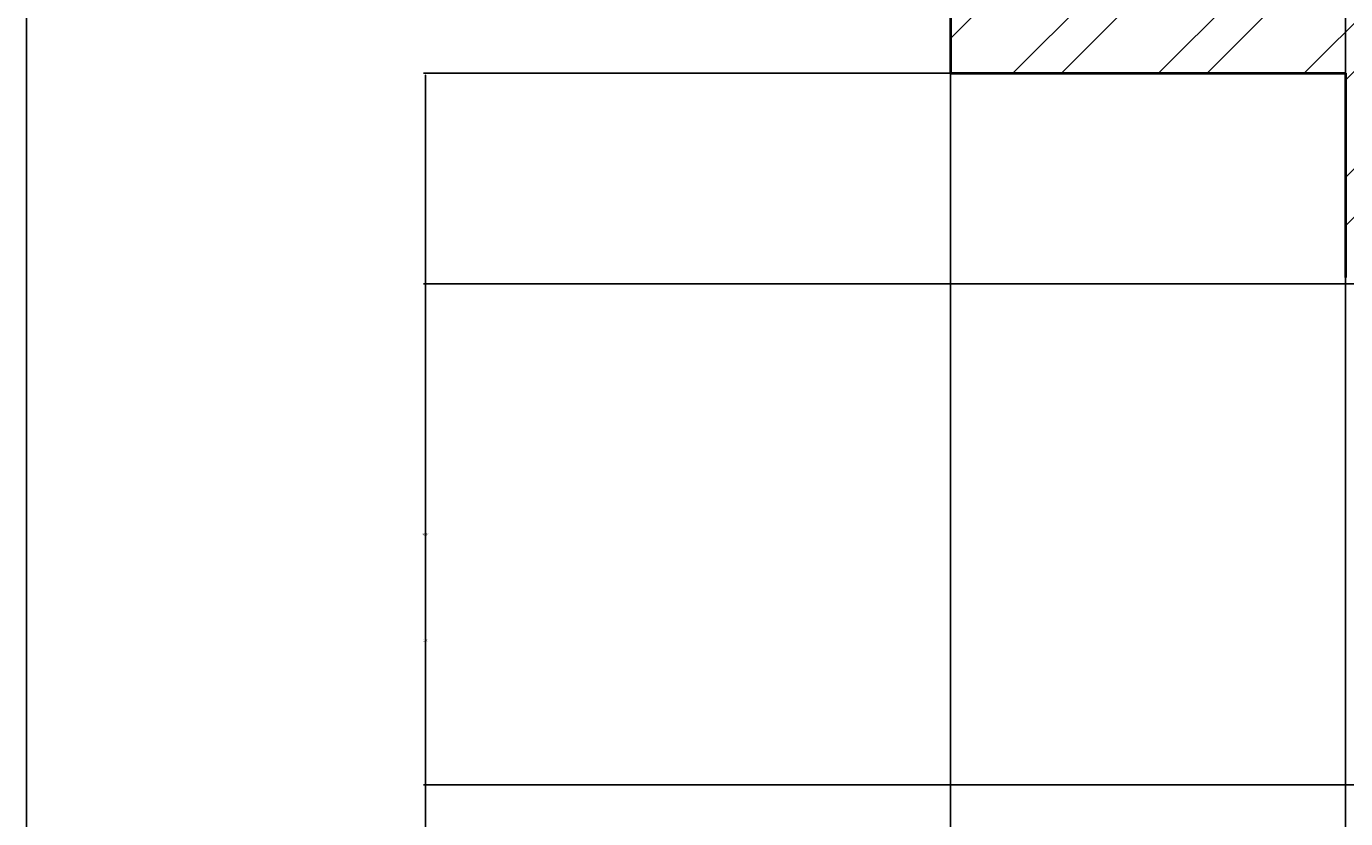
# Model space of a CAD drawing. Units: inches. Extents: x 1601 to 2297, y 1496 to 2631.
# Tile 11 of 57: x 1601 to 1723, y 2067 to 2141. Entities that reach past the tile are written whole.
import ezdxf

# ---------------------------------------------------------------- set-up
doc = ezdxf.new("R2010")
doc.units = ezdxf.units.IN
for name, color, linetype, lineweight in [('A-ANNO-DIMS', 2, 'Continuous', 18), ('A-ANNO-TTLB', 7, 'Continuous', 25), ('A-WALL', 7, 'Continuous', 40), ('A-WALL-PATT', 215, 'Continuous', 13)]:
    doc.layers.add(name, color=color, linetype=linetype, lineweight=lineweight)
doc.styles.get("Standard").update_dxf_attribs({"font": 'arial.ttf'})
doc.dimstyles.get("Standard").update_dxf_attribs({"dimtxt": 0.18, "dimasz": 0.18, "dimexe": 0.18, "dimexo": 0.0625, "dimgap": 0.09, "dimtad": 0, "dimtih": 1, "dimtoh": 1, "dimdec": 4, "dimzin": 0, "dimdsep": 46, "dimtxsty": 'Standard', "dimcen": 0.09, "dimadec": 0, "dimazin": 0, "dimtfac": 1, "dimtdec": 4, "dimtofl": 0, "dimtmove": 0, "dimatfit": 3, "dimfxl": 1, "dimtolj": 1, "dimtzin": 0, "dimarcsym": 0})

# ---------------------------------------------------------------- blocks, each defined once
blk = doc.blocks.new('*D31')
at = {"layer": 'A-ANNO-DIMS', "color": 0, "lineweight": -2, "transparency": 16777216}
for p, q in [((1685.97, 2136.33), (1637.31, 2136.33)), ((1637.49, 2136.15), (1637.49, 2084.01)), ((1637.49, 2031.51), (1637.49, 2083.64)), ((1685.97, 2031.33), (1637.31, 2031.33))]:
    blk.add_line(p, q, dxfattribs=at)
at = {"layer": 'A-ANNO-DIMS', "color": 0, "transparency": 16777216}
for points in [[(1637.46, 2136.15), (1637.52, 2136.15), (1637.49, 2136.33)], [(1637.46, 2031.51), (1637.52, 2031.51), (1637.49, 2031.33)]]:
    blk.add_solid(points, dxfattribs=at)
at = {"layer": 'Defpoints', "color": 0, "transparency": 16777216}
for p in [(1637.49, 2136.33), (1686.04, 2136.33), (1686.04, 2031.33)]:
    blk.add_point(p, dxfattribs=at)
at = {"layer": 'A-ANNO-DIMS', "color": 0, "transparency": 16777216, "insert": (1637.49, 2083.83), "char_height": 0.18, "attachment_point": 5}
blk.add_mtext('\\A1;105', dxfattribs=at)
blk = doc.blocks.new('*D32')
at = {"layer": 'A-ANNO-DIMS', "color": 0, "lineweight": -2, "transparency": 16777216}
for p, q in [((1686.04, 2031.39), (1686.04, 2581.06)), ((1722.57, 2031.39), (1722.57, 2581.06)), ((1686.22, 2580.88), (1703.91, 2580.88)), ((1722.39, 2580.88), (1704.7, 2580.88))]:
    blk.add_line(p, q, dxfattribs=at)
at = {"layer": 'A-ANNO-DIMS', "color": 0, "transparency": 16777216}
for points in [[(1686.22, 2580.91), (1686.22, 2580.85), (1686.04, 2580.88)], [(1722.39, 2580.91), (1722.39, 2580.85), (1722.57, 2580.88)]]:
    blk.add_solid(points, dxfattribs=at)
at = {"layer": 'Defpoints', "color": 0, "transparency": 16777216}
for p in [(1722.57, 2580.88), (1686.04, 2031.33), (1722.57, 2031.33)]:
    blk.add_point(p, dxfattribs=at)
at = {"layer": 'A-ANNO-DIMS', "color": 0, "transparency": 16777216, "insert": (1704.3, 2580.88), "char_height": 0.18, "attachment_point": 5}
blk.add_mtext('\\A1;36.53', dxfattribs=at)
blk = doc.blocks.new('*D36')
at = {"layer": 'A-ANNO-DIMS', "color": 0, "lineweight": -2, "transparency": 16777216}
for p, q in [((1686.04, 1635.39), (1686.04, 2581.06)), ((1739.33, 1635.39), (1739.33, 2581.06)), ((1686.22, 2580.88), (1712.36, 2580.88)), ((1739.15, 2580.88), (1713.01, 2580.88))]:
    blk.add_line(p, q, dxfattribs=at)
at = {"layer": 'A-ANNO-DIMS', "color": 0, "transparency": 16777216}
for points in [[(1686.22, 2580.91), (1686.22, 2580.85), (1686.04, 2580.88)], [(1739.15, 2580.91), (1739.15, 2580.85), (1739.33, 2580.88)]]:
    blk.add_solid(points, dxfattribs=at)
at = {"layer": 'Defpoints', "color": 0, "transparency": 16777216}
for p in [(1739.33, 2580.88), (1686.04, 1635.33), (1739.33, 1635.33)]:
    blk.add_point(p, dxfattribs=at)
at = {"layer": 'A-ANNO-DIMS', "color": 0, "transparency": 16777216, "insert": (1712.69, 2580.88), "char_height": 0.18, "attachment_point": 5}
blk.add_mtext('\\A1;53.3', dxfattribs=at)
blk = doc.blocks.new('*D44')
at = {"layer": 'A-ANNO-DIMS', "color": 0, "lineweight": -2, "transparency": 16777216}
for p, q in [((1958.97, 2116.84), (1637.31, 2116.84)), ((1637.49, 2116.66), (1637.49, 2093.85)), ((1637.49, 2070.67), (1637.49, 2093.48)), ((1958.97, 2070.49), (1637.31, 2070.49))]:
    blk.add_line(p, q, dxfattribs=at)
at = {"layer": 'A-ANNO-DIMS', "color": 0, "transparency": 16777216}
for points in [[(1637.46, 2116.66), (1637.52, 2116.66), (1637.49, 2116.84)], [(1637.46, 2070.67), (1637.52, 2070.67), (1637.49, 2070.49)]]:
    blk.add_solid(points, dxfattribs=at)
at = {"layer": 'Defpoints', "color": 0, "transparency": 16777216}
for p in [(1637.49, 2116.84), (1959.04, 2116.84), (1959.04, 2070.49)]:
    blk.add_point(p, dxfattribs=at)
at = {"layer": 'A-ANNO-DIMS', "color": 0, "transparency": 16777216, "insert": (1637.49, 2093.67), "char_height": 0.18, "attachment_point": 5}
blk.add_mtext('\\A1;46.34', dxfattribs=at)

msp = doc.modelspace()

# ---------------------------------------------------------------- hatches: boundary and pattern name
at = {"layer": 'A-WALL-PATT'}
h = msp.add_hatch(dxfattribs=at)
h.set_pattern_fill('ANSI32', color=256)
h.paths.add_polyline_path([(1973.9371, 2211.3254), (1893.0373, 2211.3254), (1893.0373, 2287.8254), (1884.6167, 2287.8254), (1884.6167, 2285.5754), (1884.6167, 2283.3254), (1888.5373, 2283.3254), (1888.5373, 2145.3254), (1695.0373, 2145.3254), (1695.0373, 2173.8724), (1690.5373, 2173.8724), (1686.0373, 2173.8724), (1686.0373, 2136.3254), (1722.5687, 2136.3254), (1722.5687, 2117.4352), (1731.5687, 2117.4352), (1731.5687, 2136.3254), (1893.0373, 2136.3254), (1893.0373, 2202.3254), (1959.0373, 2202.3254), (1959.0373, 2182.1303), (1968.0373, 2182.1303), (1968.0373, 2202.3254), (1973.9371, 2202.3254)])
h.paths.add_polyline_path([(2094.0373, 2274.6364), (2096.4294, 2274.6364), (2096.4294, 2276.8864), (2096.4294, 2279.1364), (2094.0373, 2279.1364), (2094.0373, 2290.8254), (2094.0373, 2295.3254), (2089.5373, 2295.3254), (2089.5373, 2230.8254), (2035.5373, 2230.8254), (2035.5373, 2299.8254), (2031.0373, 2299.8254), (2031.0373, 2211.3254), (2023.0065, 2211.3254), (2023.0065, 2202.3254), (2031.0373, 2202.3254), (2031.0373, 2140.8254), (1968.0373, 2140.8254), (1968.0373, 2145.9106), (1963.5373, 2145.9106), (1959.0373, 2145.9106), (1959.0373, 2116.839), (1963.5373, 2116.839), (1968.0373, 2116.839), (1968.0373, 2131.8254), (2031.0373, 2131.8254), (2031.0373, 2094.3254), (2031.0373, 2085.3254), (2031.0373, 2056.8254), (1968.0373, 2056.8254), (1968.0373, 2070.4947), (1963.5373, 2070.4947), (1959.0373, 2070.4947), (1959.0373, 2040.3029), (1968.0373, 2040.3029), (1968.0373, 2047.8254), (2031.0373, 2047.8254), (2031.0373, 1983.3254), (2031.0373, 1978.8254), (2021.1979, 1978.8254), (2021.1979, 1974.3254), (2031.0373, 1974.3254), (2031.0373, 1954.3528), (2035.5373, 1954.3528), (2035.5373, 1974.3254), (2035.5373, 1981.8254), (2055.5513, 1981.8254), (2055.5513, 1986.3254), (2035.5373, 1986.3254), (2035.5373, 2047.8254), (2040.0373, 2047.8254), (2040.0373, 2085.3254), (2040.0373, 2094.3254), (2040.0373, 2140.8254), (2035.5373, 2140.8254), (2035.5373, 2226.3254), (2089.5373, 2226.3254), (2094.0373, 2226.3254)])
h.paths.add_polyline_path([(2226.0373, 2230.8254), (2134.5373, 2230.8254), (2134.5373, 2233.5437), (2130.0373, 2233.5437), (2130.0373, 2226.3254), (2134.5373, 2226.3254), (2226.0373, 2226.3254)])
h.paths.add_polyline_path([(1807.1169, 1573.5395), (2055.0405, 1573.5395), (2055.0405, 1610.6322), (1807.1169, 1610.6322)], flags=9)
h.paths.add_polyline_path([(1841.1631, 1712.7967), (1870.3957, 1712.7967), (1870.3957, 1731.454), (1841.1631, 1731.454)], flags=9)
h.paths.add_polyline_path([(2144.3862, 1772.185), (2191.0233, 1772.185), (2191.0233, 1790.8423), (2144.3862, 1790.8423)], flags=9)
h.paths.add_polyline_path([(2143.0128, 1827.3312), (2177.9958, 1827.3312), (2177.9958, 1845.9886), (2143.0128, 1845.9886)], flags=9)
h.paths.add_polyline_path([(2041.2439, 1833.5691), (2070.8516, 1833.5691), (2070.8516, 1852.2264), (2041.2439, 1852.2264)], flags=9)
h.paths.add_polyline_path([(2097.2791, 1947.0598), (2134.2061, 1947.0598), (2134.2061, 1965.7171), (2097.2791, 1965.7171)], flags=9)
h.paths.add_polyline_path([(2214.995, 1904.3124), (2214.995, 1942.2899), (2196.3376, 1942.2899), (2196.3376, 1904.3124)], flags=9)
h.paths.add_polyline_path([(2186.6284, 2043.8031), (2219.7935, 2043.8031), (2219.7935, 2062.4605), (2186.6284, 2062.4605)], flags=9)
h.paths.add_polyline_path([(2064.0877, 2031.616), (2097.4949, 2031.616), (2097.4949, 2050.2734), (2064.0877, 2050.2734)], flags=9)
h.paths.add_polyline_path([(1973.1349, 1986.0688), (2008.4009, 1986.0688), (2008.4009, 2004.7261), (1973.1349, 2004.7261)], flags=25)
h.paths.add_polyline_path([(1976.3676, 2106.9635), (2005.7469, 2106.9635), (2005.7469, 2125.6209), (1976.3676, 2125.6209)], flags=25)
h.paths.add_polyline_path([(1991.7852, 2180.4863), (2027.0513, 2180.4863), (2027.0513, 2199.1437), (1991.7852, 2199.1437)], flags=25)
h.paths.add_polyline_path([(2106.1801, 2187.9359), (2152.2101, 2187.9359), (2152.2101, 2206.5932), (2106.1801, 2206.5932)], flags=9)
h.paths.add_polyline_path([(2148.6686, 2262.2542), (2182.318, 2262.2542), (2182.318, 2280.9115), (2148.6686, 2280.9115)], flags=9)
h.paths.add_polyline_path([(2041.6327, 2252.8147), (2071.2405, 2252.8147), (2071.2405, 2271.4721), (2041.6327, 2271.4721)], flags=25)
h.paths.add_polyline_path([(2063.9734, 2375.4265), (2100.9004, 2375.4265), (2100.9004, 2394.0839), (2063.9734, 2394.0839)], flags=9)
h.paths.add_polyline_path([(2216.4955, 2330.9748), (2216.4955, 2370.2654), (2197.8381, 2370.2654), (2197.8381, 2330.9748)], flags=9)
h.paths.add_polyline_path([(2179.1416, 2485.8687), (2212.3067, 2485.8687), (2212.3067, 2504.5261), (2179.1416, 2504.5261)], flags=9)
h.paths.add_polyline_path([(2078.7442, 2471.1516), (2112.1514, 2471.1516), (2112.1514, 2489.809), (2078.7442, 2489.809)], flags=9)
h.paths.add_polyline_path([(1915.9631, 2329.4668), (1952.8902, 2329.4668), (1952.8902, 2348.1241), (1915.9631, 2348.1241)], flags=9)
h.paths.add_polyline_path([(1904.3189, 2499.6709), (1940.4512, 2499.6709), (1940.4512, 2518.3282), (1904.3189, 2518.3282)], flags=9)
h.paths.add_polyline_path([(1892.3665, 2100.4595), (1925.6374, 2100.4595), (1925.6374, 2119.1169), (1892.3665, 2119.1169)], flags=9)
h.paths.add_polyline_path([(1909.2984, 1805.9631), (1946.2254, 1805.9631), (1946.2254, 1824.6205), (1909.2984, 1824.6205)], flags=9)
h.paths.add_polyline_path([(1934.6056, 1658.616), (1970.738, 1658.616), (1970.738, 1677.2733), (1934.6056, 1677.2733)], flags=9)
h.paths.add_polyline_path([(1711.2052, 1789.8902), (1750.0456, 1789.8902), (1750.0456, 1808.5476), (1711.2052, 1808.5476)], flags=9)
h.paths.add_polyline_path([(1742.7874, 1854.6743), (1771.9449, 1854.6743), (1771.9449, 1873.3317), (1742.7874, 1873.3317)], flags=9)
h.paths.add_polyline_path([(1807.3592, 1997.7912), (1850.1116, 1997.7912), (1850.1116, 2016.4486), (1807.3592, 2016.4486)], flags=9)
h.paths.add_polyline_path([(1717.4579, 2237.7844), (1760.2103, 2237.7844), (1760.2103, 2256.4417), (1717.4579, 2256.4417)], flags=25)
h.paths.add_polyline_path([(1780.9285, 2324.0623), (1810.086, 2324.0623), (1810.086, 2342.7197), (1780.9285, 2342.7197)], flags=9)
h.paths.add_polyline_path([(1837.696, 2449.2024), (1866.9286, 2449.2024), (1866.9286, 2467.8598), (1837.696, 2467.8598)], flags=9)
h.paths.add_polyline_path([(1712.7752, 2484.9404), (1751.6156, 2484.9404), (1751.6156, 2503.5977), (1712.7752, 2503.5977)], flags=9)

# ---------------------------------------------------------------- linework, layer by layer
at = {"layer": 'A-ANNO-TTLB'}
msp.add_lwpolyline([(1600.5933, 2631.1477), (2297.129, 2631.1477), (2297.129, 1496.1026), (1600.5933, 1496.1026)], close=True, dxfattribs=at)
at = {"layer": 'A-WALL'}
for p, q in [((1686.0373, 2173.8724), (1686.0373, 2136.3254)), ((1686.0373, 2136.3254), (1722.5687, 2136.3254)), ((1722.5687, 2136.3254), (1722.5687, 2117.4352))]:
    msp.add_line(p, q, dxfattribs=at)

# ---------------------------------------------------------------- dimensions: what is measured, and where the dimension line sits
at = {"layer": 'A-ANNO-DIMS'}
for base, p1, p2, override, picture, middle in [((1722.5687, 2580.8754), (1686.0373, 2031.3254), (1722.5687, 2031.3254), {"dimdec": 2, "dimlfac": 1, "dimrnd": 0, "dimzin": 0, "dimdsep": 46, "dimlunit": 2}, '*D32', (1704.303, 2580.8754)), ((1739.3335, 2580.8754), (1686.0373, 1635.3254), (1739.3335, 1635.3254), {"dimdec": 1, "dimlfac": 1, "dimrnd": 0, "dimzin": 0, "dimdsep": 46, "dimlunit": 2}, '*D36', (1712.6854, 2580.8754))]:
    dim = msp.add_linear_dim(base=base, p1=p1, p2=p2, dimstyle='Standard', override=override, dxfattribs=at)
    dim.commit()
    dim.dimension.update_dxf_attribs({"geometry": picture, "text_midpoint": middle})
for base, p1, p2, override, picture, middle in [((1637.4873, 2136.3254), (1686.0373, 2031.3254), (1686.0373, 2136.3254), {"dimdec": 0, "dimlfac": 1, "dimrnd": 0, "dimzin": 0, "dimdsep": 46, "dimlunit": 2}, '*D31', (1637.4873, 2083.8254)), ((1637.4873, 2116.839), (1959.0373, 2070.4947), (1959.0373, 2116.839), {"dimdec": 2, "dimlfac": 1, "dimrnd": 0, "dimzin": 0, "dimdsep": 46, "dimlunit": 2}, '*D44', (1637.4873, 2093.6668))]:
    dim = msp.add_linear_dim(base=base, p1=p1, p2=p2, angle=90, dimstyle='Standard', override=override, dxfattribs=at)
    dim.commit()
    dim.dimension.update_dxf_attribs({"geometry": picture, "text_midpoint": middle})

doc.saveas('drawing.dxf')
